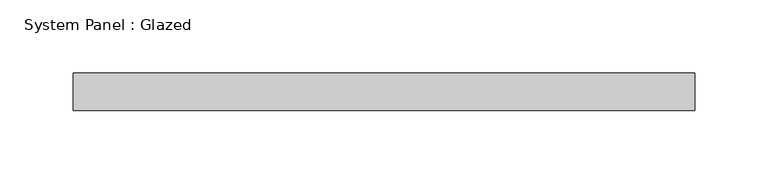
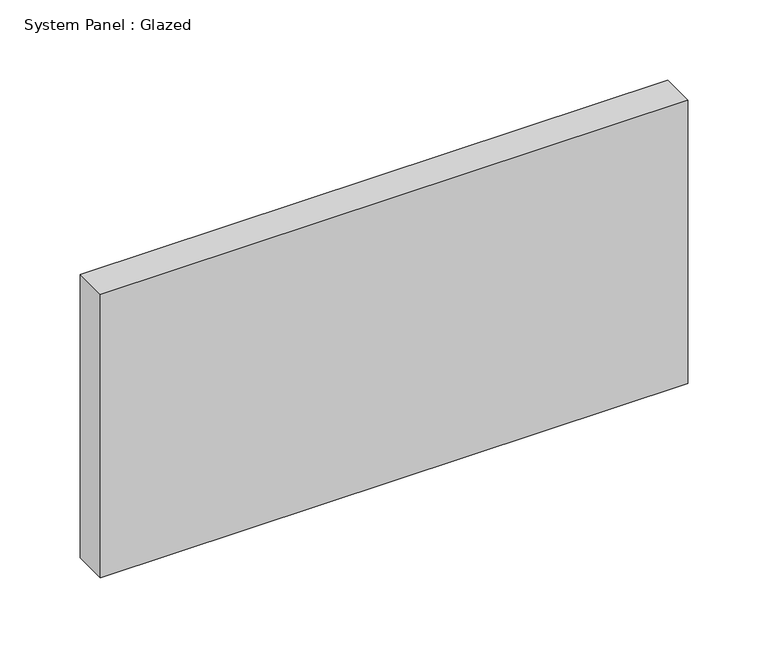
"""IFC4 building model written with IfcOpenShell, lengths in millimetres: plate geometry, System Panel : Glazed."""

from ifc_helpers import new_model, si_unit, origin, origin_with_axes, place, context, project, spatial, polyline, outline, extrude, source, transform, mapped, element, save


def system_panel_glazed_54f7da7e(model_context):
    return source(origin(), model_context, "Body", "SweptSolid", [
        extrude(outline(polyline([(211.6666667, 19.05), (-211.6666667, 19.05), (-211.6666667, 44.45), (211.6666667, 44.45), (211.6666667, 19.05)])), origin_with_axes(), (0.0, 0.0, 1.0), 215.9),
    ])


if __name__ == "__main__":
    model = new_model("IFC4")
    model_context = context("Model", 3, world=origin())
    ifc_project = project(units=[si_unit("LENGTHUNIT", "METRE", prefix="MILLI")], contexts=[model_context])
    site = spatial("IfcSite", under=ifc_project)
    building = spatial("IfcBuilding", under=site)
    placement = place(None, origin())
    system_panel_glazed_shape = system_panel_glazed_54f7da7e(model_context)
    element("IfcPlate", 1, ObjectType="System Panel : Glazed", at=placement, inside=building, context=model_context, shape_type="MappedRepresentation", body=[
        mapped(system_panel_glazed_shape, transform((0.0, 0.0, 0.0), x_axis=(1.0, 0.0, 0.0), y_axis=(0.0, 1.0, 0.0), z_axis=(0.0, 0.0, 1.0))),
    ])
    save(model, "model.ifc")

# Revit data of these elements
# Type "System Panel : Glazed"
#   Construction Type Id = "GSP4R"
#   Analytic Construction = "1/8 in Pilkington single glazing"
#   Visual Light Transmittance = 0.9
#   Solar Heat Gain Coefficient = 0.86
#   Heat Transfer Coefficient (U) = 1.18115 BTU/(h·ft²·°F)
#   Define Thermal Properties by = 1
# Element 1 (IfcPlate, "System Panel : Glazed")
#   Materials on its faces: "Glass"
# Materials
#   "Glass": class "Glass", colour RGB 0 128 192, transparency 0.75, Description = "Soda Lime Glass", Cost = 0
